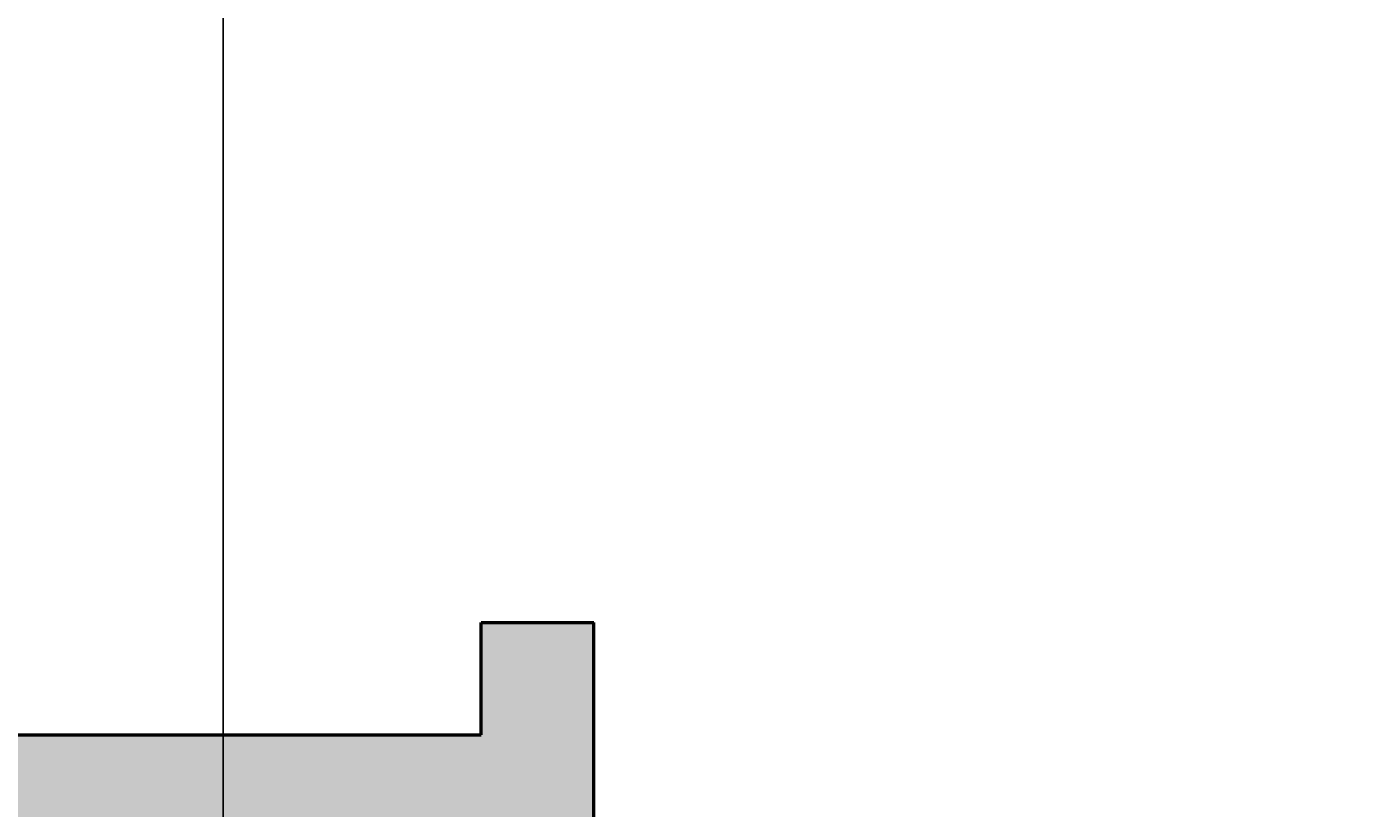
# Model space of a CAD drawing. Units: inches. Extents: x 2231 to 2461, y 2045 to 2455.
# Tile 9 of 95: x 2279 to 2326, y 2122 to 2150. Entities that reach past the tile are written whole.
import ezdxf

# ---------------------------------------------------------------- set-up
doc = ezdxf.new("R2010")
doc.units = ezdxf.units.IN
doc.layers.add('A-ANNO-DIMS', color=2, linetype='Continuous', lineweight=18)
doc.layers.add('A-WALL', color=7, linetype='Continuous', lineweight=50)
doc.layers.add('A-WALL-PATT', color=18, linetype='Continuous', lineweight=13, true_color=0x000000)
doc.styles.get("Standard").update_dxf_attribs({"font": 'arial.ttf'})
doc.dimstyles.get("Standard").update_dxf_attribs({"dimtxt": 0.18, "dimasz": 0.18, "dimexe": 0.18, "dimexo": 0.0625, "dimgap": 0.09, "dimtad": 0, "dimtih": 1, "dimtoh": 1, "dimdec": 4, "dimzin": 0, "dimdsep": 46, "dimtxsty": 'Standard', "dimcen": 0.09, "dimadec": 0, "dimazin": 0, "dimtfac": 1, "dimtdec": 4, "dimtofl": 0, "dimtmove": 0, "dimatfit": 3, "dimfxl": 1, "dimtolj": 1, "dimtzin": 0, "dimarcsym": 0})

# ---------------------------------------------------------------- blocks, each defined once
blk = doc.blocks.new('*D51')
at = {"layer": 'A-ANNO-DIMS', "color": 0, "lineweight": -2, "transparency": 16777216}
for p, q in [((2258.794, 2306.77), (2258.794, 2044.803)), ((2330.794, 2306.77), (2330.794, 2044.803)), ((2258.974, 2044.983), (2294.576, 2044.983)), ((2330.614, 2044.983), (2295.011, 2044.983))]:
    blk.add_line(p, q, dxfattribs=at)
at = {"layer": 'A-ANNO-DIMS', "color": 0, "transparency": 16777216}
for points in [[(2258.974, 2045.013), (2258.974, 2044.953), (2258.794, 2044.983)], [(2330.614, 2045.013), (2330.614, 2044.953), (2330.794, 2044.983)]]:
    blk.add_solid(points, dxfattribs=at)
at = {"layer": 'Defpoints', "color": 0, "transparency": 16777216}
for p in [(2258.794, 2306.833), (2330.794, 2306.833), (2330.794, 2044.983)]:
    blk.add_point(p, dxfattribs=at)
at = {"layer": 'A-ANNO-DIMS', "color": 0, "transparency": 16777216, "insert": (2294.794, 2044.983), "char_height": 0.18, "attachment_point": 5}
blk.add_mtext('\\A1;72', dxfattribs=at)
blk = doc.blocks.new('*D65')
at = {"layer": 'A-ANNO-DIMS', "color": 0, "lineweight": -2, "transparency": 16777216}
for p, q in [((2285.635, 2189.285), (2285.635, 2044.803)), ((2340.667, 2189.285), (2340.667, 2044.803)), ((2285.815, 2044.983), (2312.758, 2044.983)), ((2340.487, 2044.983), (2313.545, 2044.983))]:
    blk.add_line(p, q, dxfattribs=at)
at = {"layer": 'A-ANNO-DIMS', "color": 0, "transparency": 16777216}
for points in [[(2285.815, 2045.013), (2285.815, 2044.953), (2285.635, 2044.983)], [(2340.487, 2045.013), (2340.487, 2044.953), (2340.667, 2044.983)]]:
    blk.add_solid(points, dxfattribs=at)
at = {"layer": 'Defpoints', "color": 0, "transparency": 16777216}
for p in [(2285.635, 2189.348), (2340.667, 2189.348), (2340.667, 2044.983)]:
    blk.add_point(p, dxfattribs=at)
at = {"layer": 'A-ANNO-DIMS', "color": 0, "transparency": 16777216, "insert": (2313.151, 2044.983), "char_height": 0.18, "attachment_point": 5}
blk.add_mtext('\\A1;55.03', dxfattribs=at)

msp = doc.modelspace()

# ---------------------------------------------------------------- hatches: boundary and pattern name
at = {"layer": 'A-WALL-PATT'}
h = msp.add_hatch(color=256, dxfattribs=at)
h.dxf.hatch_style = 1
h.paths.add_polyline_path([(2441.7935, 2269.1535), (2432.7935, 2269.1535), (2432.7935, 2186.8328), (2396.7935, 2186.8328), (2396.7935, 2286.8328), (2394.7935, 2286.8328), (2394.7935, 2186.8328), (2334.7935, 2186.8328), (2334.7935, 2182.8328), (2432.7935, 2182.8328), (2432.7935, 2072.8328), (2416.6639, 2072.8328), (2416.6639, 2063.8328), (2441.7935, 2063.8328)])
h.paths.add_polyline_path([(2368.6639, 2072.8328), (2367.04, 2072.8328), (2330.7942, 2072.8328), (2330.7397, 2063.8328), (2368.6639, 2063.8328)])
h.paths.add_polyline_path([(2300.7392, 2068.3328), (2300.7392, 2072.8328), (2298.7935, 2072.8328), (2294.7935, 2072.8328), (2258.7935, 2072.8328), (2258.7935, 2120.8328), (2294.7935, 2120.8328), (2298.7935, 2120.8328), (2298.7935, 2128.8328), (2294.7935, 2128.8328), (2294.7935, 2124.8328), (2258.7935, 2124.8328), (2258.7935, 2182.8328), (2294.7935, 2182.8328), (2294.7935, 2174.8328), (2298.7935, 2174.8328), (2298.7935, 2182.8328), (2304.7935, 2182.8328), (2304.7935, 2186.8328), (2258.7935, 2186.8328), (2258.7935, 2221.999), (2249.7935, 2221.999), (2249.7935, 2063.8328), (2300.7392, 2063.8328)])
h.paths.add_polyline_path([(2391.9338, 2435.8328), (2333.82, 2435.8328), (2333.82, 2426.8328), (2368.7935, 2426.8328), (2368.7935, 2374.9508), (2368.7935, 2370.8328), (2372.3935, 2370.8328), (2372.7935, 2370.8328), (2372.7935, 2426.8328), (2391.9338, 2426.8328)])
h.paths.add_polyline_path([(2441.7935, 2435.8328), (2415.9338, 2435.8328), (2415.9338, 2426.8328), (2432.7935, 2426.8328), (2432.7935, 2334.8328), (2372.7935, 2334.8328), (2372.7935, 2346.8328), (2368.7935, 2346.8328), (2368.7935, 2306.8328), (2360.7935, 2306.8328), (2360.7935, 2302.8328), (2368.7935, 2302.8328), (2372.7935, 2302.8328), (2372.7935, 2330.8328), (2432.7935, 2330.8328), (2432.7935, 2317.1535), (2441.7935, 2317.1535)])
h.paths.add_polyline_path([(2285.82, 2435.8328), (2249.7935, 2435.8328), (2249.7935, 2269.999), (2258.7935, 2269.999), (2258.7935, 2302.8328), (2318.8168, 2302.8328), (2330.7935, 2302.8328), (2330.7935, 2306.8328), (2258.7935, 2306.8328), (2258.7935, 2426.8328), (2285.82, 2426.8328)])

# ---------------------------------------------------------------- linework, layer by layer
at = {"layer": 'A-WALL'}
for p, q in [((2294.7935, 2124.8328), (2294.7935, 2128.8328)), ((2294.7935, 2128.8328), (2298.7935, 2128.8328)), ((2298.7935, 2120.8328), (2298.7935, 2128.8328)), ((2258.7935, 2124.8328), (2294.7935, 2124.8328))]:
    msp.add_line(p, q, dxfattribs=at)

# ---------------------------------------------------------------- dimensions: what is measured, and where the dimension line sits
at = {"layer": 'A-ANNO-DIMS'}
for base, p1, p2, override, picture, middle in [((2330.7935, 2044.9825), (2258.7935, 2306.8328), (2330.7935, 2306.8328), {"dimdec": 0, "dimlfac": 1, "dimrnd": 0, "dimzin": 0, "dimdsep": 46, "dimlunit": 2}, '*D51', (2294.7935, 2044.9825)), ((2340.6673, 2044.9825), (2285.6353, 2189.3477), (2340.6673, 2189.3477), {"dimdec": 2, "dimlfac": 1, "dimrnd": 0, "dimzin": 0, "dimdsep": 46, "dimlunit": 2}, '*D65', (2313.1513, 2044.9825))]:
    dim = msp.add_linear_dim(base=base, p1=p1, p2=p2, dimstyle='Standard', override=override, dxfattribs=at)
    dim.commit()
    dim.dimension.update_dxf_attribs({"geometry": picture, "text_midpoint": middle})

doc.saveas('drawing.dxf')
